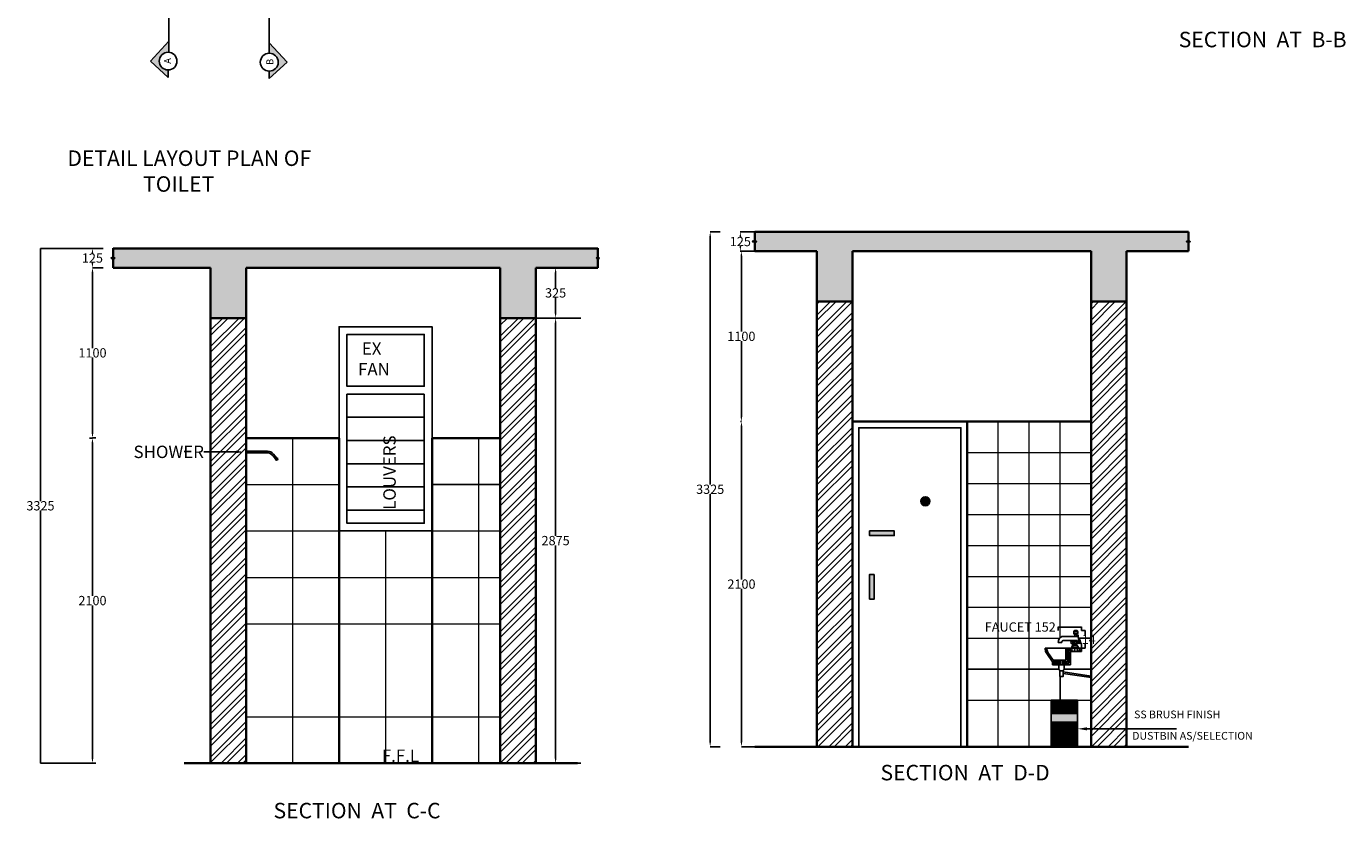
# Model space of a CAD drawing. Units: millimetres. Extents: x -2204 to 11247, y -2365 to 12631.
# Tile 1 of 3: x -294 to 8225, y -2365 to 2752. Entities that reach past the tile are written whole.
import ezdxf
from ezdxf import colors
from ezdxf.entities.mleader import LeaderData, LeaderLine
from ezdxf.math import Vec2, Vec3

# ---------------------------------------------------------------- set-up
doc = ezdxf.new("R2010")
doc.units = ezdxf.units.MM
doc.header["$MEASUREMENT"] = 0
for name, color, linetype, lineweight in [('A-ANNO-DIMS', 2, 'Continuous', 18), ('A-ANNO-SYMB', 2, 'Continuous', 25), ('A-ANNO-TEXT', 7, 'Continuous', 18), ('A-DOOR', 4, 'Continuous', 25), ('A-ELEV-PATT', 9, 'Continuous', 13), ('A-EQPM', 6, 'Continuous', 25), ('A-FLOR-FIXT', 8, 'Continuous', 25), ('A-SECT', 7, 'Continuous', 35), ('A-SECT-PATT', 252, 'Continuous', 18), ('A-WALL-PATT', 8, 'Continuous', 18)]:
    doc.layers.add(name, color=color, linetype=linetype, lineweight=lineweight)
doc.styles.get("Standard").update_dxf_attribs({"font": 'arial.ttf'})
doc.dimstyles.get("Standard").update_dxf_attribs({"dimtxt": 60, "dimasz": 0.18, "dimexe": 0.18, "dimexo": 0.0625, "dimgap": 0.09, "dimtad": 0, "dimtih": 1, "dimtoh": 1, "dimdec": 0, "dimzin": 0, "dimdsep": 46, "dimtxsty": 'Standard', "dimcen": 0.09, "dimadec": 0, "dimazin": 0, "dimtfac": 1, "dimtdec": 0, "dimtofl": 0, "dimtmove": 0, "dimatfit": 3, "dimfxl": 1, "dimtolj": 1, "dimtzin": 0, "dimarcsym": 0})

# ---------------------------------------------------------------- blocks, each defined once
blk = doc.blocks.new('*D3')
at = {"layer": 'A-ANNO-DIMS', "color": 0, "lineweight": -2, "transparency": 16777216}
for p, q in [((2996, 1193.4), (3124.1, 1193.4)), ((3123.9, 1163.4), (3123.9, 1061.6)), ((3123.9, 898.4), (3123.9, 1000.1)), ((2996, 868.4), (3124.1, 868.4))]:
    blk.add_line(p, q, dxfattribs=at)
at = {"layer": 'A-ANNO-DIMS', "color": 0, "transparency": 16777216}
for points in [[(3118.9, 1163.4), (3128.9, 1163.4), (3123.9, 1193.4)], [(3118.9, 898.4), (3128.9, 898.4), (3123.9, 868.4)]]:
    blk.add_solid(points, dxfattribs=at)
at = {"layer": 'Defpoints', "color": 0, "transparency": 16777216}
for p in [(2995.9, 1193.4), (2995.9, 868.4), (3123.9, 868.4)]:
    blk.add_point(p, dxfattribs=at)
at = {"layer": 'A-ANNO-DIMS', "color": 0, "transparency": 16777216, "insert": (3123.9, 1030.9), "char_height": 60, "attachment_point": 5}
blk.add_mtext('\\A1;325', dxfattribs=at)
blk = doc.blocks.new('*D4')
at = {"layer": 'A-ANNO-DIMS', "color": 0, "lineweight": -2, "transparency": 16777216}
for p, q in [((3285.9, 868.4), (3123.7, 868.4)), ((3123.9, 838.4), (3123.9, -538.4)), ((3123.9, -1976.6), (3123.9, -599.8)), ((3285.9, -2006.6), (3123.7, -2006.6))]:
    blk.add_line(p, q, dxfattribs=at)
at = {"layer": 'A-ANNO-DIMS', "color": 0, "transparency": 16777216}
for points in [[(3118.9, 838.4), (3128.9, 838.4), (3123.9, 868.4)], [(3118.9, -1976.6), (3128.9, -1976.6), (3123.9, -2006.6)]]:
    blk.add_solid(points, dxfattribs=at)
at = {"layer": 'Defpoints', "color": 0, "transparency": 16777216}
for p in [(3123.9, 868.4), (3286, 868.4), (3286, -2006.6)]:
    blk.add_point(p, dxfattribs=at)
at = {"layer": 'A-ANNO-DIMS', "color": 0, "transparency": 16777216, "insert": (3123.9, -569.1), "char_height": 60, "attachment_point": 5}
blk.add_mtext('\\A1;2875', dxfattribs=at)
blk = doc.blocks.new('*D8')
at = {"layer": 'A-ANNO-DIMS', "color": 0, "lineweight": -2, "transparency": 16777216}
for p, q in [((202.4, 1318.4), (132.7, 1318.4)), ((132.9, 1288.4), (132.9, 1286.6)), ((202.4, 1193.4), (132.7, 1193.4)), ((132.9, 1223.4), (132.9, 1225.2))]:
    blk.add_line(p, q, dxfattribs=at)
at = {"layer": 'A-ANNO-DIMS', "color": 0, "transparency": 16777216}
for points in [[(127.9, 1288.4), (137.9, 1288.4), (132.9, 1318.4)], [(127.9, 1223.4), (137.9, 1223.4), (132.9, 1193.4)]]:
    blk.add_solid(points, dxfattribs=at)
at = {"layer": 'Defpoints', "color": 0, "transparency": 16777216}
for p in [(132.9, 1318.4), (202.5, 1318.4), (202.5, 1193.4)]:
    blk.add_point(p, dxfattribs=at)
at = {"layer": 'A-ANNO-DIMS', "color": 0, "transparency": 16777216, "insert": (132.9, 1255.9), "char_height": 60, "attachment_point": 5}
blk.add_mtext('\\A1;125', dxfattribs=at)
blk = doc.blocks.new('*D9')
at = {"layer": 'A-ANNO-DIMS', "color": 0, "lineweight": -2, "transparency": 16777216}
for p, q in [((133, 1193.6), (133.5, 1193.6)), ((133.3, 1163.6), (133.3, 674.2)), ((133.3, 123.4), (133.3, 612.8)), ((113.2, 93.4), (133.5, 93.4))]:
    blk.add_line(p, q, dxfattribs=at)
at = {"layer": 'A-ANNO-DIMS', "color": 0, "transparency": 16777216}
for points in [[(128.3, 1163.6), (138.3, 1163.6), (133.3, 1193.6)], [(128.3, 123.4), (138.3, 123.4), (133.3, 93.4)]]:
    blk.add_solid(points, dxfattribs=at)
at = {"layer": 'Defpoints', "color": 0, "transparency": 16777216}
for p in [(132.9, 1193.6), (133.3, 1193.6), (113.1, 93.4)]:
    blk.add_point(p, dxfattribs=at)
at = {"layer": 'A-ANNO-DIMS', "color": 0, "transparency": 16777216, "insert": (133.3, 643.5), "char_height": 60, "attachment_point": 5}
blk.add_mtext('\\A1;1100', dxfattribs=at)
blk = doc.blocks.new('*D10')
at = {"layer": 'A-ANNO-DIMS', "color": 0, "lineweight": -2, "transparency": 16777216}
for p, q in [((154.5, 93.6), (133.1, 93.6)), ((133.2, 63.6), (133.2, -925.8)), ((133.2, -1976.6), (133.2, -987.2)), ((154.5, -2006.6), (133.1, -2006.6))]:
    blk.add_line(p, q, dxfattribs=at)
at = {"layer": 'A-ANNO-DIMS', "color": 0, "transparency": 16777216}
for points in [[(128.2, 63.6), (138.2, 63.6), (133.2, 93.6)], [(128.2, -1976.6), (138.2, -1976.6), (133.2, -2006.6)]]:
    blk.add_solid(points, dxfattribs=at)
at = {"layer": 'Defpoints', "color": 0, "transparency": 16777216}
for p in [(133.2, 93.6), (154.5, 93.6), (154.5, -2006.6)]:
    blk.add_point(p, dxfattribs=at)
at = {"layer": 'A-ANNO-DIMS', "color": 0, "transparency": 16777216, "insert": (133.2, -956.5), "char_height": 60, "attachment_point": 5}
blk.add_mtext('\\A1;2100', dxfattribs=at)
blk = doc.blocks.new('*D11')
at = {"layer": 'A-ANNO-DIMS', "color": 0, "lineweight": -2, "transparency": 16777216}
for p, q in [((132.8, 1318.4), (-202.9, 1318.4)), ((-202.7, 1318.2), (-202.7, -313.4)), ((-202.7, -2006.4), (-202.7, -374.9)), ((143.7, -2006.6), (-202.9, -2006.6))]:
    blk.add_line(p, q, dxfattribs=at)
at = {"layer": 'A-ANNO-DIMS', "color": 0, "transparency": 16777216}
for points in [[(-202.7, 1318.2), (-202.6, 1318.2), (-202.7, 1318.4)], [(-202.7, -2006.4), (-202.6, -2006.4), (-202.7, -2006.6)]]:
    blk.add_solid(points, dxfattribs=at)
at = {"layer": 'Defpoints', "color": 0, "transparency": 16777216}
for p in [(132.9, 1318.4), (-202.7, -2006.6), (143.8, -2006.6)]:
    blk.add_point(p, dxfattribs=at)
at = {"layer": 'A-ANNO-DIMS', "color": 0, "transparency": 16777216, "insert": (-202.7, -344.1), "char_height": 60, "attachment_point": 5}
blk.add_mtext('\\A1;3325', dxfattribs=at)
blk = doc.blocks.new('Faucet - Bathroom side')
for p, q in [((-0.625, 4.25), (0.375, 4.25)), ((0.375, 3.75), (-0.625, 3.75)), ((-0.375, 3), (-0.375, 3.5)), ((0.125, 3.5), (0.125, 3)), ((-1.625, 0), (-1.375, 0)), ((-1.375, 0), (1.375, 0)), ((-0.88366, 0.25), (0.88424, 0.25)), ((-0.625, 3), (3.375, 3)), ((-0.375, 1.625), (-0.625, 1.625)), ((-0.375, 1.375), (-0.625, 1.375)), ((0.48078, 0.75), (-0.47286, 0.75)), ((2.875, 2), (0.375, 2)), ((0.375, 1.625), (0.625, 1.625)), ((0.375, 1.375), (0.625, 1.375)), ((4.375, 1.5), (3.375, 1.5))]:
    blk.add_line(p, q)
for points in [[(-0.625, 3.75), (-0.625, 4.25)], [(-0.375, 4.5), (0.125, 4.5)], [(0.125, 3.5), (-0.375, 3.5)], [(0.375, 4.25), (0.375, 3.75)]]:
    blk.add_lwpolyline(points)
blk.add_lwpolyline([(-0.375, 1), (-0.375, 2), (0.375, 2), (0.375, 1)], close=True)
for centre in [(-0.875, 1.5), (0, 1.5), (0.875, 1.5)]:
    blk.add_circle(centre, 0.27951)
for centre, radius, start, end in [((-0.38253, 4.2575), 0.24259, 88.22243, 181.7776), ((-0.38253, 3.7424), 0.24259, 178.2224, 271.7776), ((0.13252, 4.2575), 0.24259, 358.2224, 91.77757), ((0.13252, 3.7424), 0.24259, 268.2224, 1.777565), ((3.45929, -0.0281), 5.08436, 143.4467, 179.6834), ((-1.75, 1.375), 1.42522, 285.2551, 344.7449), ((1.75, 1.375), 1.42522, 195.2551, 254.7449), ((-2.49562, -0.286), 3.38273, 9.709485, 29.48735), ((2.96867, 1.5936), 0.41699, 347.0192, 102.9808), ((2.70708, 1.4714), 1.66816, 0.9827695, 66.39737)]:
    blk.add_arc(centre, radius, start, end)
blk = doc.blocks.new('*D15')
at = {"layer": 'A-ANNO-DIMS', "color": 0, "lineweight": -2, "transparency": 16777216}
for p, q in [((4411.2, 1425), (4316.6, 1425)), ((4316.8, 1395), (4316.8, 1393.2)), ((4411.2, 1300), (4316.6, 1300)), ((4316.8, 1330), (4316.8, 1331.7))]:
    blk.add_line(p, q, dxfattribs=at)
at = {"layer": 'A-ANNO-DIMS', "color": 0, "transparency": 16777216}
for points in [[(4311.8, 1395), (4321.8, 1395), (4316.8, 1425)], [(4311.8, 1330), (4321.8, 1330), (4316.8, 1300)]]:
    blk.add_solid(points, dxfattribs=at)
at = {"layer": 'Defpoints', "color": 0, "transparency": 16777216}
for p in [(4411.3, 1425), (4316.8, 1300), (4411.3, 1300)]:
    blk.add_point(p, dxfattribs=at)
at = {"layer": 'A-ANNO-DIMS', "color": 0, "transparency": 16777216, "insert": (4316.8, 1362.5), "char_height": 60, "attachment_point": 5}
blk.add_mtext('\\A1;125', dxfattribs=at)
blk = doc.blocks.new('*D16')
at = {"layer": 'A-ANNO-DIMS', "color": 0, "lineweight": -2, "transparency": 16777216}
for p, q in [((4316.9, 1300.1), (4323.5, 1300.1)), ((4323.4, 1270.1), (4323.4, 780.8)), ((4323.4, 230), (4323.4, 719.3)), ((4316.9, 200), (4323.5, 200))]:
    blk.add_line(p, q, dxfattribs=at)
at = {"layer": 'A-ANNO-DIMS', "color": 0, "transparency": 16777216}
for points in [[(4318.4, 1270.1), (4328.4, 1270.1), (4323.4, 1300.1)], [(4318.4, 230), (4328.4, 230), (4323.4, 200)]]:
    blk.add_solid(points, dxfattribs=at)
at = {"layer": 'Defpoints', "color": 0, "transparency": 16777216}
for p in [(4316.8, 1300.1), (4316.8, 200), (4323.4, 200)]:
    blk.add_point(p, dxfattribs=at)
at = {"layer": 'A-ANNO-DIMS', "color": 0, "transparency": 16777216, "insert": (4323.4, 750.1), "char_height": 60, "attachment_point": 5}
blk.add_mtext('\\A1;1100', dxfattribs=at)
blk = doc.blocks.new('*D17')
at = {"layer": 'A-ANNO-DIMS', "color": 0, "lineweight": -2, "transparency": 16777216}
for p, q in [((4323.6, 200), (4324.2, 200)), ((4324, 170), (4324, -819.3)), ((4324, -1870), (4324, -880.8)), ((4411.2, -1900), (4323.8, -1900))]:
    blk.add_line(p, q, dxfattribs=at)
at = {"layer": 'A-ANNO-DIMS', "color": 0, "transparency": 16777216}
for points in [[(4319, 170), (4329, 170), (4324, 200)], [(4319, -1870), (4329, -1870), (4324, -1900)]]:
    blk.add_solid(points, dxfattribs=at)
at = {"layer": 'Defpoints', "color": 0, "transparency": 16777216}
for p in [(4323.5, 200), (4324, 200), (4411.3, -1900)]:
    blk.add_point(p, dxfattribs=at)
at = {"layer": 'A-ANNO-DIMS', "color": 0, "transparency": 16777216, "insert": (4324, -850), "char_height": 60, "attachment_point": 5}
blk.add_mtext('\\A1;2100', dxfattribs=at)
blk = doc.blocks.new('*D18')
at = {"layer": 'A-ANNO-DIMS', "color": 0, "lineweight": -2, "transparency": 16777216}
for p, q in [((4185.9, 1425), (4121.9, 1425)), ((4122, 1395), (4122, -206.8)), ((4122, -1870), (4122, -268.3)), ((4185.9, -1900), (4121.9, -1900))]:
    blk.add_line(p, q, dxfattribs=at)
at = {"layer": 'A-ANNO-DIMS', "color": 0, "transparency": 16777216}
for points in [[(4117, 1395), (4127, 1395), (4122, 1425)], [(4117, -1870), (4127, -1870), (4122, -1900)]]:
    blk.add_solid(points, dxfattribs=at)
at = {"layer": 'Defpoints', "color": 0, "transparency": 16777216}
for p in [(4185.9, 1425), (4122, -1900), (4185.9, -1900)]:
    blk.add_point(p, dxfattribs=at)
at = {"layer": 'A-ANNO-DIMS', "color": 0, "transparency": 16777216, "insert": (4122, -237.5), "char_height": 60, "attachment_point": 5}
blk.add_mtext('\\A1;3325', dxfattribs=at)
blk = doc.blocks.new('*D30')
at = {"layer": 'A-ANNO-DIMS', "color": 0, "lineweight": -2, "transparency": 16777216}
for p, q in [((6368.3, -1127.1), (6368.1, -1127.1)), ((6368.3, -1149.9), (6368.3, -1127)), ((6520.5, -1127.1), (6368.5, -1127.1)), ((6520.7, -1149.9), (6520.7, -1127))]:
    blk.add_line(p, q, dxfattribs=at)
at = {"layer": 'A-ANNO-DIMS', "color": 0, "transparency": 16777216}
for points in [[(6368.5, -1127.1), (6368.5, -1127.2), (6368.3, -1127.1)], [(6520.5, -1127.1), (6520.5, -1127.2), (6520.7, -1127.1)]]:
    blk.add_solid(points, dxfattribs=at)
at = {"layer": 'Defpoints', "color": 0, "transparency": 16777216}
for p in [(6368.3, -1127.1), (6368.3, -1150), (6520.7, -1150)]:
    blk.add_point(p, dxfattribs=at)
at = {"layer": 'A-ANNO-DIMS', "color": 0, "transparency": 16777216, "insert": (6124.5, -1127.1), "char_height": 60, "attachment_point": 5}
blk.add_mtext('\\A1;FAUCET 152', dxfattribs=at)
blk = doc.blocks.new('*D31')
at = {"layer": 'A-ANNO-DIMS', "color": 0, "lineweight": -2, "transparency": 16777216}
for p, q in [((6520.8, -1150), (6543.7, -1150)), ((6543.6, -1150.2), (6543.6, -1177)), ((6520.8, -1264.3), (6543.7, -1264.3)), ((6543.6, -1264.2), (6543.6, -1237.4))]:
    blk.add_line(p, q, dxfattribs=at)
at = {"layer": 'A-ANNO-DIMS', "color": 0, "transparency": 16777216}
for points in [[(6543.5, -1150.2), (6543.6, -1150.2), (6543.6, -1150)], [(6543.5, -1264.2), (6543.6, -1264.2), (6543.6, -1264.3)]]:
    blk.add_solid(points, dxfattribs=at)
at = {"layer": 'Defpoints', "color": 0, "transparency": 16777216}
for p in [(6520.7, -1150), (6543.6, -1150), (6520.7, -1264.3)]:
    blk.add_point(p, dxfattribs=at)
at = {"layer": 'A-ANNO-DIMS', "color": 0, "transparency": 16777216, "insert": (6543.6, -1207.2), "char_height": 60, "attachment_point": 5}
blk.add_mtext('\\A1;114', dxfattribs=at)

msp = doc.modelspace()

# ---------------------------------------------------------------- hatches: boundary and pattern name
at = {"layer": 'A-ANNO-SYMB'}
h = msp.add_hatch(color=256, dxfattribs=at)
h.dxf.hatch_style = 1
h.paths.add_polyline_path([(507.8, 2527.6), (621.7, 2651), (621.7, 2584.8, 0.414214), (564.4, 2527.6, 0.414214), (621.7, 2470.4), (621.7, 2422.5)])
h = msp.add_hatch(color=256, dxfattribs=at)
h.dxf.hatch_style = 1
h.paths.add_polyline_path([(1389.6, 2520.5), (1274.8, 2644.9), (1274.8, 2578.2, -0.414214), (1332.5, 2520.5, -0.414214), (1274.8, 2462.8), (1274.8, 2414.5)])
at = {"layer": 'A-DOOR'}
h = msp.add_hatch(color=256, dxfattribs=at)
h.dxf.hatch_style = 1
h.paths.add_polyline_path([(5482.7, -314.6, 1), (5540.9, -314.6, 1)])
h = msp.add_hatch(color=256, dxfattribs=at)
h.dxf.hatch_style = 1
h.paths.add_polyline_path([(5181.8, -787.2), (5151.8, -787.2), (5151.8, -946.3), (5181.8, -946.3)])
h.paths.add_polyline_path([(5310.9, -506.7), (5151.8, -506.7), (5151.8, -536.7), (5310.9, -536.7)])
at = {"layer": 'A-FLOR-FIXT'}
h = msp.add_hatch(color=256, dxfattribs=at)
h.dxf.hatch_style = 1
h.paths.add_polyline_path([(1330.1, -41.8, 1), (1314.4, -41.8, 1)])
h.paths.add_polyline_path([(1317.4, -41.8, -1), (1327.1, -41.8, -1)], flags=16)
h.paths.add_polyline_path([(1318.3, -39.8), (1319.3, -39.8), (1319.3, -38.8), (1320.3, -38.8), (1320.3, -37.8), (1324.3, -37.8), (1324.3, -38.8), (1325.3, -38.8), (1325.3, -44.8), (1324.3, -44.8), (1324.3, -45.8), (1320.3, -45.8), (1320.3, -44.8), (1319.3, -44.8), (1319.3, -43.8), (1318.3, -43.8)], flags=0)
h.paths.add_polyline_path([(1321.3, -42.8), (1321.3, -40.8), (1323.3, -40.8), (1323.3, -42.8)], flags=0)
h = msp.add_hatch(color=256, dxfattribs=at)
h.dxf.hatch_style = 1
h.paths.add_polyline_path([(6494.9, -1685.4), (6322.9, -1685.4), (6322.9, -1741.7), (6494.9, -1741.7)])
at = {"layer": 'A-SECT-PATT'}
h = msp.add_hatch(dxfattribs=at)
h.set_pattern_fill('AR-SAND', color=256, scale=10)
h.paths.add_polyline_path([(5041.3, 1300), (6581.3, 1300), (6581.3, 975), (6811.3, 975), (6811.3, 1300), (7211.3, 1300), (7211.3, 1425), (4411.3, 1425), (4411.3, 1300), (4811.3, 1300), (4811.3, 975), (5041.3, 975)])
h = msp.add_hatch(dxfattribs=at)
h.set_pattern_fill('AR-SAND', color=256, scale=10)
h.paths.add_polyline_path([(3395.9, 1318.4), (265.9, 1318.4), (265.9, 1193.4), (895.9, 1193.4), (895.9, 868.4), (1125.9, 868.4), (1125.9, 1193.4), (2765.9, 1193.4), (2765.9, 868.4), (2995.9, 868.4), (2995.9, 1193.4), (3395.9, 1193.4)])
at = {"layer": 'A-WALL-PATT'}
h = msp.add_hatch(dxfattribs=at)
h.set_pattern_fill('ANSI32', color=256, scale=200)
h.paths.add_polyline_path([(5041.3, 975), (4811.3, 975), (4811.3, -1900), (5041.3, -1900), (5041.3, 200)])
h.paths.add_polyline_path([(6811.3, 975), (6581.3, 975), (6581.3, -1900), (6811.3, -1900)])
h = msp.add_hatch(dxfattribs=at)
h.set_pattern_fill('ANSI32', color=256, scale=200)
h.paths.add_polyline_path([(2995.9, 868.4), (2765.9, 868.4), (2765.9, -2006.6), (2995.9, -2006.6)])
h.paths.add_polyline_path([(1125.9, 868.4), (895.9, 868.4), (895.9, -2006.6), (1125.9, -2006.6)])

# ---------------------------------------------------------------- linework, layer by layer
at = {"layer": 'A-ANNO-SYMB'}
for p, q in [((1274.8, 8209.7), (1274.8, 2578.2)), ((626.2, 4500.1), (626.2, 2584.7)), ((507.8, 2527.6), (626.2, 2655.9)), ((1389.6, 2520.5), (1274.8, 2644.9)), ((507.8, 2527.6), (621.7, 2422.5)), ((1389.6, 2520.5), (1274.8, 2414.5)), ((621.7, 2470.4), (621.7, 2422.5)), ((1274.8, 2462.8), (1274.8, 2414.5))]:
    msp.add_line(p, q, dxfattribs=at)
for centre, radius in [((621.7, 2527.6), 57.2), ((1274.8, 2520.5), 57.7)]:
    msp.add_circle(centre, radius, dxfattribs=at)
at = {"layer": 'A-DOOR'}
msp.add_lwpolyline([(5081.3, -1900), (5081.3, 160), (5741.3, 160), (5741.3, -1900)], dxfattribs=at)
for points in [[(5151.8, -506.7), (5310.9, -506.7), (5310.9, -536.7), (5151.8, -536.7)], [(5181.8, -787.2), (5181.8, -946.3), (5151.8, -946.3), (5151.8, -787.2)]]:
    msp.add_lwpolyline(points, close=True, dxfattribs=at)
msp.add_circle((5511.8, -314.6), 29.1, dxfattribs=at)
at = {"layer": 'A-ELEV-PATT'}
for p, q in [((5781.3, -1900), (5781.3, 200)), ((5981.3, -1900), (5981.3, 200)), ((6181.3, -1900), (6181.3, 200)), ((6381.3, -1196.4), (6381.3, 200)), ((1425.9, 93.4), (1425.9, -2006.6)), ((2625.9, 93.4), (2625.9, -2006.6)), ((5781.3, 0), (6581.3, 0)), ((1125.9, -206.6), (1725.9, -206.6)), ((5781.3, -200), (6581.3, -200)), ((5781.3, -400), (6581.3, -400)), ((1125.9, -506.6), (2765.9, -506.6)), ((2025.9, -506.6), (2025.9, -2006.6)), ((5781.3, -600), (6581.3, -600)), ((1125.9, -806.6), (2765.9, -806.6)), ((5781.3, -800), (6581.3, -800)), ((5781.3, -1000), (6581.3, -1000)), ((1125.9, -1106.6), (2765.9, -1106.6)), ((5781.3, -1200), (6378, -1200)), ((5781.3, -1600), (6581.3, -1600)), ((1125.9, -1706.6), (2765.9, -1706.6))]:
    msp.add_line(p, q, dxfattribs=at)
at = {"layer": 'A-EQPM'}
msp.add_line((2325.9, -206.6), (2765.9, -206.6), dxfattribs=at)
for points in [[(2325.9, -506.6), (1725.9, -506.6), (1725.9, 812), (2325.9, 812)], [(1775.9, 762), (2275.9, 762), (2275.9, 427.5), (1775.9, 427.5)]]:
    msp.add_lwpolyline(points, close=True, dxfattribs=at)
for points in [[(1725.9, 377.5), (1725.9, 812), (2325.9, 812), (2325.9, 377.5)], [(1775.9, 427.5), (1775.9, 762), (2275.9, 762), (2275.9, 427.5)], [(2275.9, 377.5), (2275.9, -456.6), (1775.9, -456.6), (1775.9, 377.5)], [(2275.9, 377.5), (1775.9, 377.5)]]:
    msp.add_lwpolyline(points, dxfattribs=at)
at = {"layer": 'A-EQPM', "ltscale": 3}
for points in [[(2275.9, 227.5), (1775.9, 227.5)], [(2275.9, 77.5), (1775.9, 77.5)], [(2275.9, -72.5), (1775.9, -72.5)], [(2275.9, -222.5), (1775.9, -222.5)], [(2275.9, -372.5), (1775.9, -372.5)]]:
    msp.add_lwpolyline(points, dxfattribs=at)
at = {"layer": 'A-FLOR-FIXT'}
for p, q in [((1125.9, 8.5), (1263.7, 8.5)), ((1125.9, -1.5), (1259, -1.5)), ((1297.7, -19.8), (1314.6, -40.4)), ((1302.4, -9.8), (1322.2, -34)), ((1317.4, -41.8), (1327.1, -41.8)), ((1317.5, -40.8), (1327, -40.8)), ((1317.5, -42.8), (1327, -42.8)), ((1317.9, -39.8), (1326.7, -39.8)), ((1317.9, -43.8), (1326.7, -43.8)), ((1318.3, -44.6), (1318.3, -39.1)), ((1318.5, -38.8), (1326.1, -38.8)), ((1318.5, -44.8), (1326.1, -44.8)), ((1319.3, -45.7), (1319.3, -38)), ((1319.5, -37.8), (1325, -37.8)), ((1319.5, -45.8), (1325, -45.8)), ((1320.3, -46.3), (1320.3, -37.4)), ((1321.3, -46.6), (1321.3, -37.1)), ((1322.3, -46.7), (1322.3, -37)), ((1323.3, -46.6), (1323.3, -37.1)), ((1324.3, -46.3), (1324.3, -37.4)), ((1325.3, -45.7), (1325.3, -38)), ((6444.5, -1264.3), (6286, -1264.3)), ((6286, -1264.3), (6286, -1269.3)), ((6418.4, -1341.1), (6418.4, -1264.3)), ((6428.4, -1351.1), (6428.4, -1264.3)), ((6438.4, -1361.1), (6438.4, -1264.3)), ((6503.1, -1200), (6581.3, -1200)), ((6520.7, -1264.3), (6520.7, -1286)), ((6295, -1298), (6332.1, -1351.1)), ((6303.2, -1292.3), (6337.4, -1341.1)), ((6332.1, -1351.1), (6385, -1351.1)), ((6332.1, -1371.1), (6332.1, -1351.1)), ((6332.1, -1361.1), (6385, -1361.1)), ((6337.4, -1341.1), (6418.4, -1341.1)), ((6397.4, -1351.1), (6428.4, -1351.1)), ((6397.4, -1361.1), (6438.4, -1361.1)), ((6520.7, -1286), (6448.4, -1286)), ((6448.4, -1371.1), (6448.4, -1286)), ((5781.3, -1400), (6373.5, -1400)), ((6332.1, -1371.1), (6448.4, -1371.1)), ((6381.3, -1685.4), (6381.3, -1447.5)), ((6400.7, -1417.6), (6582.7, -1444)), ((6400.7, -1427.7), (6581.3, -1453.9)), ((6407.9, -1400), (6581.3, -1400))]:
    msp.add_line(p, q, dxfattribs=at)
for points in [[(6385, -1371.1), (6397.4, -1371.1), (6397.4, -1341.1), (6385, -1341.1)], [(6322.9, -1600), (6494.9, -1600), (6494.9, -1900), (6322.9, -1900)], [(6322.9, -1685.4), (6494.9, -1685.4), (6494.9, -1741.7), (6322.9, -1741.7)]]:
    msp.add_lwpolyline(points, close=True, dxfattribs=at)
for points in [[(6373.3, -1399.4), (6373.3, -1371.1), (6408.1, -1371.1), (6408.1, -1399.4)], [(6400.7, -1407.8), (6400.7, -1447.5), (6380, -1447.5), (6380, -1407.8)], [(6332.9, -1685.4), (6332.9, -1600)], [(6342.9, -1685.4), (6342.9, -1600)], [(6352.9, -1685.4), (6352.9, -1600)], [(6362.9, -1685.4), (6362.9, -1600)], [(6372.9, -1685.4), (6372.9, -1600)], [(6382.9, -1685.4), (6382.9, -1600)], [(6392.9, -1685.4), (6392.9, -1600)], [(6402.9, -1685.4), (6402.9, -1600)], [(6414.9, -1600), (6414.9, -1685.4)], [(6424.9, -1600), (6424.9, -1685.4)], [(6434.9, -1600), (6434.9, -1685.4)], [(6444.9, -1600), (6444.9, -1685.4)], [(6454.9, -1600), (6454.9, -1685.4)], [(6464.9, -1600), (6464.9, -1685.4)], [(6474.9, -1600), (6474.9, -1685.4)], [(6484.9, -1600), (6484.9, -1685.4)], [(6332.9, -1900), (6332.9, -1741.7)], [(6342.9, -1900), (6342.9, -1741.7)], [(6352.9, -1900), (6352.9, -1741.7)], [(6362.9, -1900), (6362.9, -1741.7)], [(6372.9, -1900), (6372.9, -1741.7)], [(6382.9, -1900), (6382.9, -1741.7)], [(6392.9, -1900), (6392.9, -1741.7)], [(6402.9, -1900), (6402.9, -1741.7)], [(6414.9, -1741.7), (6414.9, -1900)], [(6424.9, -1741.7), (6424.9, -1900)], [(6434.9, -1741.7), (6434.9, -1900)], [(6444.9, -1741.7), (6444.9, -1900)], [(6454.9, -1741.7), (6454.9, -1900)], [(6464.9, -1741.7), (6464.9, -1900)], [(6474.9, -1741.7), (6474.9, -1900)], [(6484.9, -1741.7), (6484.9, -1900)]]:
    msp.add_lwpolyline(points, dxfattribs=at)
for centre, radius in [((1322.3, -41.8), 7.86), ((1322.3, -41.8), 4.86), ((6452.9, -1274.2), 6.18), ((6484.5, -1275.8), 10.1), ((6511.4, -1274.3), 6.18)]:
    msp.add_circle(centre, radius, dxfattribs=at)
for centre, radius, start, end in [((1263.7, -41.5), 50, 39.36116, 90), ((1259, -51.5), 50, 39.36116, 90), ((6336, -1269.3), 50, 180, 214.95919), ((6336, -1269.3), 40, 172.82215, 214.95919), ((6390.7, -1392.3), 18.8, 202.1314, 337.8686)]:
    msp.add_arc(centre, radius, start, end, dxfattribs=at)
at = {"layer": 'A-SECT'}
for p, q in [((4411.3, 1425), (7211.3, 1425)), ((4411.3, 1425), (4411.3, 1367.4)), ((7211.3, 1366.6), (7211.3, 1425)), ((265.9, 1318.4), (3395.9, 1318.4)), ((265.9, 1318.4), (265.9, 1259.7)), ((3395.9, 1318.4), (3395.9, 1257.5)), ((4411.3, 1357.5), (4411.3, 1300)), ((4411.3, 1300), (4811.3, 1300)), ((4811.3, 1300), (4811.3, -1900)), ((5041.3, 1300), (5041.3, -1900)), ((5041.3, 1300), (6581.3, 1300)), ((6581.3, -1900), (6581.3, 1300)), ((6811.3, -1900), (6811.3, 1300)), ((6811.3, 1300), (7211.3, 1300)), ((7211.3, 1300), (7211.3, 1356.4)), ((265.9, 1252.4), (265.9, 1193.4)), ((265.9, 1193.4), (895.9, 1193.4)), ((895.9, 1193.4), (895.9, -2006.6)), ((1125.9, 1193.4), (1125.9, -2006.6)), ((1125.9, 1193.4), (2765.9, 1193.4)), ((2765.9, 1193.4), (2765.9, -2006.6)), ((2995.9, 1193.4), (2995.9, -2006.6)), ((2995.9, 1193.4), (3395.9, 1193.4)), ((3395.9, 1253.9), (3395.9, 1193.4)), ((4811.3, 975), (5041.3, 975)), ((6581.3, 975), (6811.3, 975)), ((895.9, 868.4), (1125.9, 868.4)), ((2765.9, 868.4), (2995.9, 868.4)), ((5041.3, 200), (6581.3, 200)), ((1125.9, 93.4), (1725.9, 93.4)), ((1725.9, 93.4), (1725.9, -2006.6)), ((2325.9, 93.4), (2325.9, -2006.6)), ((2325.9, 93.4), (2765.9, 93.4)), ((4811.3, -1900), (4411.3, -1900)), ((4811.3, -1900), (6811.3, -1900)), ((6811.3, -1900), (7211.3, -1900)), ((895.9, -2006.6), (724.9, -2006.6)), ((895.9, -2006.6), (2995.9, -2006.6)), ((2995.9, -2006.6), (3265, -2006.6))]:
    msp.add_line(p, q, dxfattribs=at)
for points in [[(4411.3, 1425.1), (4411.3, 1367.4), (4395.3, 1362.6), (4421.1, 1362.3), (4411.3, 1357.5), (4411.3, 1299.8)], [(7211.3, 1425.1), (7211.3, 1366.6), (7199.2, 1362.6), (7219.6, 1362.3), (7211.3, 1356.4), (7211.3, 1299.8)], [(265.9, 1318.6), (265.9, 1259.7), (254.4, 1256), (276.2, 1255.8), (265.9, 1252.4), (265.9, 1193.2)], [(3395.9, 1318.6), (3395.9, 1257.5), (3388.5, 1256), (3404.5, 1255.8), (3395.9, 1253.9), (3395.9, 1193.2)]]:
    msp.add_lwpolyline(points, dxfattribs=at)
msp.add_lwpolyline([(5041.3, 200), (5781.3, 200), (5781.3, -1900), (5041.3, -1900)], close=True, dxfattribs=at)

# ---------------------------------------------------------------- block references
at = {"layer": 'A-FLOR-FIXT', "xscale": -25.4, "yscale": 25.4, "zscale": 25.4}
msp.add_blockref('Faucet - Bathroom side', (6479.4, -1264.3), dxfattribs=at)

# ---------------------------------------------------------------- texts
at = {"layer": 'A-ANNO-SYMB', "rotation": 90}
for s, width, gutter_width, insert, char_height, attachment_point in [('A', 63.028, 0.443, (639.9, 2510.3), 44.3, 7), ('B', 63.548, 0.447, (1256.4, 2503.1), 44.7, 1)]:
    msp.add_mtext_dynamic_manual_height_columns(s, width=width, gutter_width=gutter_width, heights=[0], dxfattribs=dict(at, insert=insert, char_height=char_height, attachment_point=attachment_point))
at = {"layer": 'A-ANNO-TEXT', "attachment_point": 1}
for s, width, insert, char_height in [('{\\fArial|b1|i0|c0|p34;SECTION  AT  B-B}', 2816.974, (7147.7, 2717), 100), ('\\pxt8;{\\fArial|b1|i0|c0|p34;DETAIL LAYOUT PLAN OF\\P                TOILET}', 2816.974, (-28.8, 1950.6), 100), ('{\\H0.8x;      EX\\P     FAN}', 820.155, (1725.9, 711), 100), ('SS BRUSH FINISH', 2816.974, (6859.3, -1666.8), 50), ('DUSTBIN AS/SELECTION', 2816.974, (6847.3, -1804.8), 50), ('{\\H0.8x;     F.F.L}', 820.155, (1879.3, -1918.3), 100), ('{\\fArial|b1|i0|c0|p34;SECTION  AT  D-D}', 2816.974, (5221.9, -2017.5), 100), ('{\\fArial|b1|i0|c0|p34;SECTION  AT  C-C}', 2816.974, (1302.5, -2262.9), 100)]:
    msp.add_mtext_dynamic_manual_height_columns(s, width=width, gutter_width=1, heights=[0], dxfattribs=dict(at, insert=insert, char_height=char_height))
at = {"layer": 'A-ANNO-TEXT', "insert": (2011.5, -370.2), "char_height": 100, "attachment_point": 1, "rotation": 90}
msp.add_mtext_dynamic_manual_height_columns('{\\H0.8x;LOUVERS}', width=820.155, gutter_width=1, heights=[0], dxfattribs=at)

# ---------------------------------------------------------------- dimensions: what is measured, and where the dimension line sits
at = {"layer": 'A-ANNO-DIMS'}
for base, p1, p2, override, picture, middle in [((4122, -1900), (4185.9, 1425), (4185.9, -1900), {"dimasz": 30, "dimclrd": 0, "dimclre": 0, "dimclrt": 0}, '*D18', (4122, -237.5)), ((4316.8, 1300), (4411.3, 1425), (4411.3, 1300), {"dimasz": 30, "dimclrd": 0, "dimclre": 0, "dimclrt": 0}, '*D15', (4316.8, 1362.5)), ((-202.7, -2006.6), (132.9, 1318.4), (143.8, -2006.6), {"dimclrd": 0, "dimclre": 0, "dimclrt": 0}, '*D11', (-202.7, -344.1)), ((132.9, 1318.4), (202.5, 1193.4), (202.5, 1318.4), {"dimasz": 30, "dimclrd": 0, "dimclre": 0, "dimclrt": 0}, '*D8', (132.9, 1255.9)), ((4323.4, 200), (4316.8, 1300.1), (4316.8, 200), {"dimasz": 30, "dimclrd": 0, "dimclre": 0, "dimclrt": 0}, '*D16', (4323.4, 750.1)), ((133.3, 1193.6), (113.1, 93.4), (132.9, 1193.6), {"dimasz": 30, "dimclrd": 0, "dimclre": 0, "dimclrt": 0}, '*D9', (133.3, 643.5)), ((3123.9, 868.4), (2995.9, 1193.4), (2995.9, 868.4), {"dimasz": 30, "dimclrd": 0, "dimclre": 0, "dimclrt": 0}, '*D3', (3123.9, 1030.9)), ((3123.9, 868.4), (3286, -2006.6), (3286, 868.4), {"dimasz": 30, "dimclrd": 0, "dimclre": 0, "dimclrt": 0}, '*D4', (3123.9, -569.1)), ((4324, 200), (4411.3, -1900), (4323.5, 200), {"dimasz": 30, "dimclrd": 0, "dimclre": 0, "dimclrt": 0}, '*D17', (4324, -850)), ((133.2, 93.6), (154.5, -2006.6), (154.5, 93.6), {"dimasz": 30, "dimclrd": 0, "dimclre": 0, "dimclrt": 0}, '*D10', (133.2, -956.5)), ((6543.6, -1150), (6520.7, -1264.3), (6520.7, -1150), {"dimdec": 0, "dimlfac": 1, "dimrnd": 0, "dimzin": 0, "dimdsep": 46, "dimlunit": 2}, '*D31', (6543.6, -1207.2))]:
    dim = msp.add_linear_dim(base=base, p1=p1, p2=p2, angle=90, dimstyle='Standard', override=override, dxfattribs=at)
    dim.commit()
    dim.dimension.update_dxf_attribs({"geometry": picture, "text_midpoint": middle})
dim = msp.add_linear_dim(base=(6368.3, -1127.1), p1=(6520.7, -1150), p2=(6368.3, -1150), angle=180, text='FAUCET <>', dimstyle='Standard', override={"dimdec": 0, "dimlfac": 1, "dimrnd": 0, "dimzin": 0, "dimdsep": 46, "dimlunit": 2}, dxfattribs=at)
dim.commit()
dim.dimension.update_dxf_attribs({"geometry": '*D30', "text_midpoint": (6124.5, -1127.1)})

# ---------------------------------------------------------------- leaders
at = {"layer": 'A-ANNO-TEXT'}
ml = msp.add_multileader_mtext('Standard', dxfattribs=at)
ml.set_content('SHOWER', color=256)
ml.set_leader_properties()
ml.build(insert=Vec2(0, 0))
ml.multileader.update_dxf_attribs({"dogleg_length": 0.36, "arrow_head_size": 50})
ctx = ml.context
ctx.base_point, ctx.char_height, ctx.arrow_head_size, ctx.landing_gap_size, ctx.plane_origin = Vec3(356.6, 3.4), 80, 50, 0.09, Vec3(1110.5, 3.4)
ctx.text_align_type = 2
notes = []
notes.append((ctx, [(0, (1, 1, 0), (853.7, 3.4), (-1, 0), 0.36, [(0, [(1110.5, 3.4)], 0, [])])]))
ctx.mtext.insert, ctx.mtext.alignment, ctx.mtext.flow_direction = Vec3(853.2, 44.1), 3, 5
ml = msp.add_multileader_mtext('Standard', dxfattribs=at)
ml.set_content('', color=256)
ml.set_leader_properties()
ml.build(insert=Vec2(0, 0))
ml.multileader.update_dxf_attribs({"dogleg_length": 0.36, "arrow_head_size": 0.18})
ctx = ml.context
ctx.base_point, ctx.char_height, ctx.arrow_head_size, ctx.landing_gap_size, ctx.plane_origin = Vec3(770.7, 5.4), 0.18, 0.18, 0.09, Vec3(725.5, 5.4)
notes.append((ctx, [(0, (1, 1, 0), (770.4, 5.4), (1, 0), 0.36, [(0, [(725.5, 5.4)], 0, [])])]))
ctx.mtext.insert, ctx.mtext.flow_direction = Vec3(770.8, 5.5), 5
ml = msp.add_multileader_mtext('Standard', dxfattribs=at)
ml.set_content('', color=256)
ml.set_leader_properties()
ml.build(insert=Vec2(0, 0))
ml.multileader.update_dxf_attribs({"dogleg_length": 0.36, "arrow_head_size": 60})
ctx = ml.context
ctx.base_point, ctx.char_height, ctx.arrow_head_size, ctx.landing_gap_size, ctx.plane_origin = Vec3(7132.1, -1784.8), 0.18, 60, 0.09, Vec3(6494.9, -1784.8)
notes.append((ctx, [(0, (1, 1, 0), (7131.8, -1784.8), (1, 0), 0.36, [(0, [(6494.9, -1784.8)], 0, [])])]))
ctx.mtext.insert, ctx.mtext.flow_direction = Vec3(7132.2, -1784.7), 5
for ctx, leaders in notes:
    for number, flags, end, landing, length, lines in leaders:
        leader = LeaderData()
        leader.index, (leader.has_last_leader_line, leader.has_dogleg_vector, leader.attachment_direction) = number, flags
        leader.last_leader_point, leader.dogleg_vector, leader.dogleg_length = Vec3(end), Vec3(landing), length
        for number, points, colour, breaks in lines:
            line = LeaderLine()
            line.index, line.vertices, line.color, line.breaks = number, Vec3.list(points), colors.encode_raw_color(colour), breaks
            leader.lines.append(line)
        ctx.leaders.append(leader)

doc.saveas('drawing.dxf')
